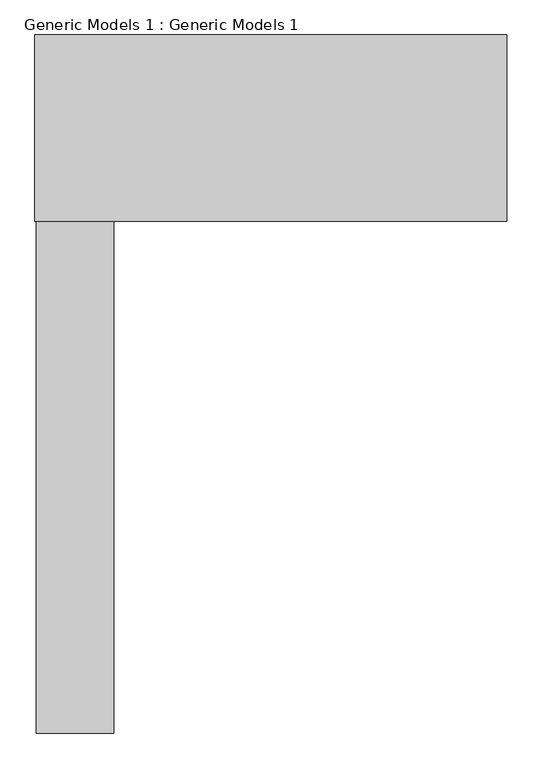
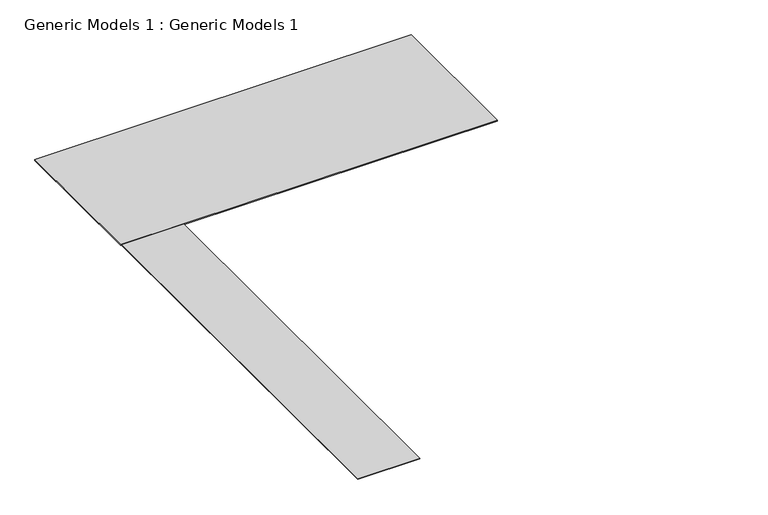
"""IFC4 building model written with IfcOpenShell, lengths in millimetres: proxy geometry, Generic Models 1 : Generic Models 1."""

from ifc_helpers import new_model, si_unit, origin, origin_with_axes, place, context, project, spatial, polyline, outline, extrude, source, transform, mapped, element, save


def generic_models_1_generic_models_1_08f91587(model_context):
    return source(origin(), model_context, "Body", "SweptSolid", [
        extrude(outline(polyline([(-15386.2175224, -16534.2384042), (-15386.2175224, 28520.0932954), (-8564.1734018, 28520.0932954), (-8564.1734018, -16534.2384042), (-15386.2175224, -16534.2384042)])), origin_with_axes(), (0.0, 0.0, 1.0), 97.7473468),
        extrude(outline(polyline([(26004.7759659, 28520.0932954), (-15524.2240341, 28520.0932954), (-15524.2240341, 44907.5461341), (26004.7759659, 44907.5461341), (26004.7759659, 28520.0932954)])), origin_with_axes(), (0.0, 0.0, 1.0), 130.0114773),
    ])


if __name__ == "__main__":
    model = new_model("IFC4")
    model_context = context("Model", 3, world=origin())
    ifc_project = project(units=[si_unit("LENGTHUNIT", "METRE", prefix="MILLI")], contexts=[model_context])
    site = spatial("IfcSite", under=ifc_project)
    building = spatial("IfcBuilding", under=site)
    placement = place(None, origin())
    generic_models_1_generic_models_1_shape = generic_models_1_generic_models_1_08f91587(model_context)
    element("IfcBuildingElementProxy", 1, Name="Generic Models 1 : Generic Models 1", ObjectType="Generic Models 1 : Generic Models 1", at=placement, inside=building, context=model_context, shape_type="MappedRepresentation", body=[
        mapped(generic_models_1_generic_models_1_shape, transform((0.0, 0.0, 0.0), x_axis=(1.0, 0.0, 0.0), y_axis=(0.0, 1.0, 0.0), z_axis=(0.0, 0.0, 1.0))),
    ])
    save(model, "model.ifc")
